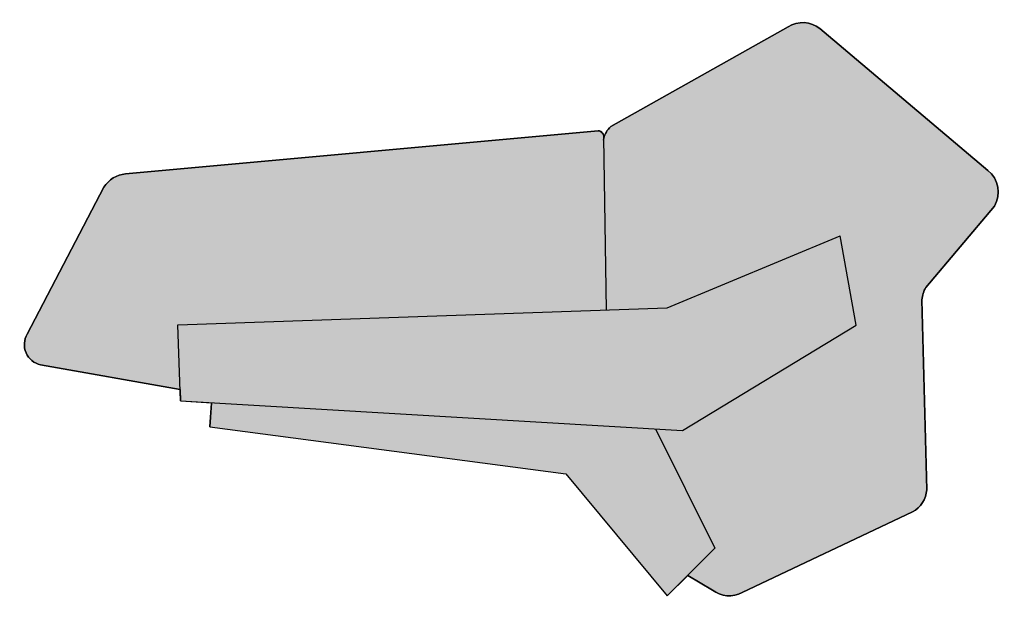
# Model space of a CAD drawing. Units: inches. Extents: x -466983 to 1020, y 324 to 318697.
# Tile 1 of 97: x -466983 to -462682, y 316138 to 318697. Entities that reach past the tile are written whole.
import ezdxf

# ---------------------------------------------------------------- set-up
doc = ezdxf.new("R2010")
doc.units = ezdxf.units.IN
doc.header["$MEASUREMENT"] = 0
doc.layers.add('A-ANNO-TTLB', color=7, linetype='Continuous', lineweight=25)
doc.layers.add('K-Hatch', color=7, linetype='Continuous')

# ---------------------------------------------------------------- blocks, each defined once
blk = doc.blocks.new('CBV_05')
at = {"layer": 'K-Hatch'}
h = blk.add_hatch(color=256, dxfattribs=at)
h.dxf.hatch_style = 1
h.paths.add_polyline_path([(614, 437), (1251.4, 62.5), (1198.3, -263.2), (564.8, -9.8), (344.4, -5.5), (343.7, -629.7, 0.159768), (369.9, -672.6), (1020.5, -1025.6, 0.317347), (1135.5, -1017.7), (1739.5, -492.7, 0.378101), (1761.2, -362.2), (1507.4, -70.4, -0.119239), (1492.6, -25.8), (1499.5, 665.1, 0.256804), (1446.2, 745.4), (822.7, 1028.7, 0.297137), (714, 1018.3), (625, 963.6), (549.5, 1037.1), (186.8, 587.5), (-1106.2, 397.7), (-1098.6, 311.5), (-1098.4, 310.2)])
h.paths.add_polyline_path([(344.4, -5.5), (-1216.9, 24.6), (-1212.3, 260), (-1718.1, 162.7, 0.51466), (-1765.1, 50), (-1478.1, -479.5, 0.244482), (-1398.8, -526.6), (323.6, -658.2, 0.453292), (343.1, -629.8, 0.006511), (343.7, -631.8)])
h = blk.add_hatch(color=256, dxfattribs=at)
h.dxf.hatch_style = 1
h.paths.add_polyline_path([(614, 437), (-1211.5, 301.9), (-1212.3, 260), (-1216.9, 24.6), (564.8, -9.8), (1198.3, -263.2), (1251.4, 62.5)])
for p, q in [((186.8, 587.5), (549.5, 1037.1)), ((725.2, 866.1), (549.5, 1037.1)), ((517.5, 431), (725.2, 866.1)), ((-1106.2, 397.7), (186.8, 587.5)), ((-1211.5, 301.9), (614, 437)), ((614, 437), (1251.4, 62.5)), ((-1106.2, 397.7), (-1098.6, 311.5)), ((-1211.5, 301.9), (-1216.9, 24.6)), ((1251.4, 62.5), (1198.3, -263.2)), ((-1216.9, 24.6), (564.8, -9.8)), ((564.8, -9.8), (1198.3, -263.2))]:
    blk.add_line(p, q)
blk.add_lwpolyline([(1761.2, -362.2, -0.378101), (1739.5, -492.7), (1135.5, -1017.7, -0.317347), (1020.5, -1025.6), (369.9, -672.6, -0.159481), (343.2, -630.1, -0.449095), (323.6, -658.2), (-1398.8, -526.6, -0.244482), (-1478.1, -479.5), (-1765.1, 50, -0.51466), (-1718.1, 162.7), (-1212.3, 260), (-1211.5, 301.9), (-1098.4, 310.2), (-1106.2, 397.7), (186.8, 587.5), (549.5, 1037.1), (625, 963.6), (714, 1018.3, -0.297137), (822.7, 1028.7), (1446.2, 745.4, -0.256804), (1499.5, 665.1), (1492.6, -25.8, 0.119239), (1507.4, -70.4)], format="xyb", close=True)
for points in [[(369.9, -672.6), (1020.5, -1025.6, 0.317347), (1135.5, -1017.7), (1739.5, -492.7, 0.378101), (1761.2, -362.2), (1507.4, -70.4, -0.119239), (1492.6, -25.8), (1499.5, 665.1, 0.256804), (1446.2, 745.4), (822.7, 1028.7, 0.297137), (714, 1018.3), (625, 963.6)], [(-1212.3, 260), (-1718.1, 162.7, 0.51466), (-1765.1, 50), (-1478.1, -479.5, 0.244482), (-1398.8, -526.6), (323.6, -658.2)]]:
    blk.add_lwpolyline(points, format="xyb")
blk.add_lwpolyline([(344.4, -5.5), (343.7, -632.6)])
for centre, radius, start, end in [((320.9, -635.5), 22.9, 276.7908, 7.9615), ((422.2, -611.1), 80.7, 188.9571, 229.6497)]:
    blk.add_arc(centre, radius, start, end)

msp = doc.modelspace()

# ---------------------------------------------------------------- block references
at = {"layer": 'A-ANNO-TTLB', "xscale": -1.200000000069848, "yscale": 1.200000000069848, "zscale": 1.199999999999999, "rotation": 180.8588529634455}
msp.add_blockref('CBV_05', (-464832.5, 317417.5), dxfattribs=at)

doc.saveas('drawing.dxf')
